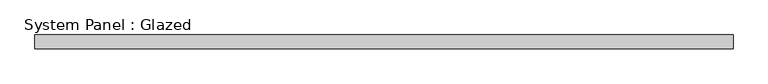
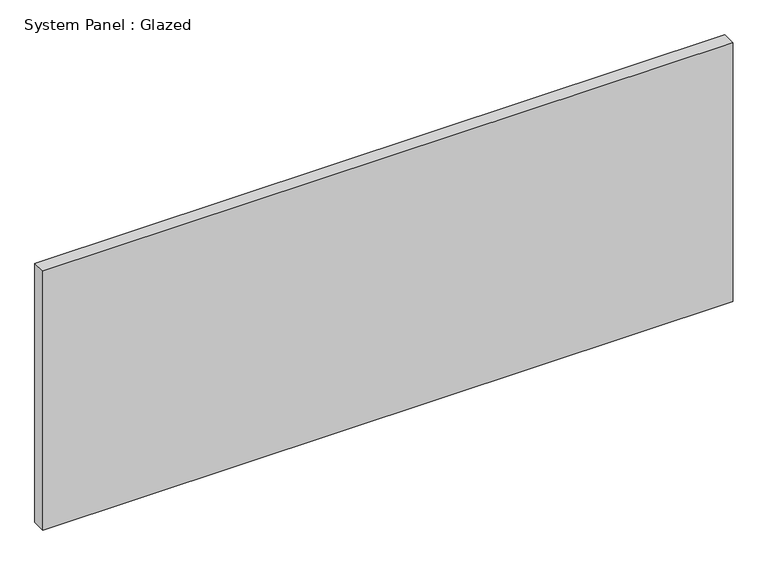
"""IFC4 building model written with IfcOpenShell, lengths in millimetres: plate geometry, System Panel : Glazed."""

from ifc_helpers import new_model, si_unit, origin, origin_with_axes, place, context, project, spatial, polyline, outline, extrude, source, transform, mapped, element, save


def system_panel_glazed_3ed2553b(model_context):
    return source(origin(), model_context, "Body", "SweptSolid", [
        extrude(outline(polyline([(647.7, 19.05), (-647.7, 19.05), (-647.7, 44.45), (647.7, 44.45), (647.7, 19.05)])), origin_with_axes(), (0.0, 0.0, 1.0), 514.35),
    ])


if __name__ == "__main__":
    model = new_model("IFC4")
    model_context = context("Model", 3, world=origin())
    ifc_project = project(units=[si_unit("LENGTHUNIT", "METRE", prefix="MILLI")], contexts=[model_context])
    site = spatial("IfcSite", under=ifc_project)
    building = spatial("IfcBuilding", under=site)
    placement = place(None, origin())
    system_panel_glazed_shape = system_panel_glazed_3ed2553b(model_context)
    element("IfcPlate", 1, ObjectType="System Panel : Glazed", at=placement, inside=building, context=model_context, shape_type="MappedRepresentation", body=[
        mapped(system_panel_glazed_shape, transform((0.0, 0.0, 0.0), x_axis=(1.0, 0.0, 0.0), y_axis=(0.0, 1.0, 0.0), z_axis=(0.0, 0.0, 1.0))),
    ])
    save(model, "model.ifc")

# Revit data of these elements
# Type "System Panel : Glazed"
#   Construction Type Id = "GSP4R"
#   Analytic Construction = "1/8 in Pilkington single glazing"
#   Visual Light Transmittance = 0.9
#   Solar Heat Gain Coefficient = 0.86
#   Heat Transfer Coefficient (U) = 1.18115 BTU/(h·ft²·°F)
# Element 1 (IfcPlate, "System Panel : Glazed")
#   Materials on its faces: "Glass"
# Materials
#   "Glass": class "Glass", colour RGB 0 128 192, transparency 0.75, Description = "Soda Lime Glass", Cost = 0
